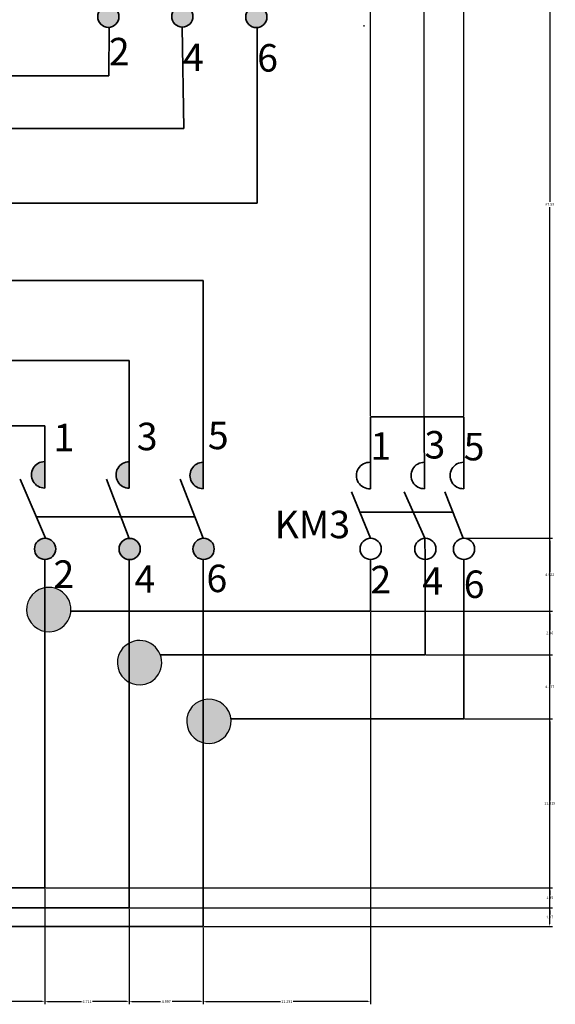
# Model space of a CAD drawing. Units: inches. Extents: x 237 to 313, y 343 to 451.
# Tile 2 of 6: x 277 to 313, y 343 to 410. Entities that reach past the tile are written whole.
import ezdxf

# ---------------------------------------------------------------- set-up
doc = ezdxf.new("R2010")
doc.units = ezdxf.units.IN
doc.header["$MEASUREMENT"] = 0
doc.layers.get('0').update_dxf_attribs({"color": 240})
for name, color, linetype, lineweight in [('A-ANNO-DIMS', 2, 'Continuous', 18), ('E-ANNO-TEXT', 7, 'Continuous', 25), ('E-DEVC', 4, 'Continuous', 35), ('E-PATT', 8, 'Continuous', 13), ('E-WIRE', 7, 'Continuous', 35), ('E-WIRE-JUNC', 7, 'Continuous', 25)]:
    doc.layers.add(name, color=color, linetype=linetype, lineweight=lineweight)
doc.styles.get("Standard").update_dxf_attribs({"font": 'arial.ttf'})
doc.dimstyles.get("Standard").update_dxf_attribs({"dimtxt": 0.18, "dimasz": 0.18, "dimexe": 0.18, "dimexo": 0.0625, "dimgap": 0.09, "dimtad": 0, "dimtih": 1, "dimtoh": 1, "dimdec": 4, "dimzin": 0, "dimdsep": 46, "dimtxsty": 'Standard', "dimcen": 0.09, "dimadec": 0, "dimazin": 0, "dimtfac": 1, "dimtdec": 4, "dimtofl": 0, "dimtmove": 0, "dimatfit": 3, "dimfxl": 1, "dimtolj": 1, "dimtzin": 0, "dimarcsym": 0})

# ---------------------------------------------------------------- blocks, each defined once
blk = doc.blocks.new('CONTACTOR-3P-NO')
h = blk.add_hatch(color=256)
h.dxf.hatch_style = 1
h.paths.add_polyline_path([(1.637, 4.965, 1), (1.637, 3.177)])
h.paths.add_polyline_path([(6.637, 4.953, 1), (6.637, 3.166)])
h.paths.add_polyline_path([(11.637, 4.931, 1), (11.637, 3.144)])
h = blk.add_hatch(color=256)
h.dxf.hatch_style = 1
h.paths.add_polyline_path([(2.354, 0.734, 1), (0.92, 0.734, 1)])
h.paths.add_polyline_path([(5.92, 0.749, 1), (7.354, 0.749, 1)])
h.paths.add_polyline_path([(10.92, 0.717, 1), (12.354, 0.717, 1)])
for p, q in [((1.414, 1.415), (0, 3.965)), ((6.423, 1.433), (4.991, 3.965)), ((11.461, 1.412), (9.739, 3.965))]:
    blk.add_line(p, q)
for centre in [(1.637, 0.734), (6.637, 0.749), (11.637, 0.717)]:
    blk.add_circle(centre, 0.717)
for centre in [(1.637, 4.071), (6.637, 4.06), (11.637, 4.037)]:
    blk.add_arc(centre, 0.894, 90, 270)
blk = doc.blocks.new('*D3')
at = {"layer": 'A-ANNO-DIMS', "color": 0, "lineweight": -2, "transparency": 16777216}
for p, q in [((242.3, 363.785), (242.3, 451.078)), ((242.48, 450.898), (274.084, 450.898)), ((306.476, 450.898), (274.872, 450.898)), ((306.656, 382.738), (306.656, 451.078))]:
    blk.add_line(p, q, dxfattribs=at)
at = {"layer": 'A-ANNO-DIMS', "color": 0, "lineweight": 35, "transparency": 16777216}
for points in [[(242.48, 450.928), (242.48, 450.868), (242.3, 450.898)], [(306.476, 450.928), (306.476, 450.868), (306.656, 450.898)]]:
    blk.add_solid(points, dxfattribs=at)
at = {"layer": 'Defpoints', "color": 0, "lineweight": 35, "transparency": 16777216}
for p in [(306.656, 450.898), (306.656, 382.675), (242.3, 363.723)]:
    blk.add_point(p, dxfattribs=at)
at = {"layer": 'A-ANNO-DIMS', "color": 0, "transparency": 16777216, "insert": (274.478, 450.898), "char_height": 0.18, "attachment_point": 5}
blk.add_mtext('\\A1;64.36', dxfattribs=at)
blk = doc.blocks.new('*D4')
at = {"layer": 'A-ANNO-DIMS', "color": 0, "lineweight": -2, "transparency": 16777216}
for p, q in [((258.115, 445.823), (312.65, 445.823)), ((312.47, 445.643), (312.47, 397.21)), ((312.47, 348.414), (312.47, 396.846)), ((289.124, 348.234), (312.65, 348.234))]:
    blk.add_line(p, q, dxfattribs=at)
at = {"layer": 'A-ANNO-DIMS', "color": 0, "lineweight": 35, "transparency": 16777216}
for points in [[(312.44, 445.643), (312.5, 445.643), (312.47, 445.823)], [(312.44, 348.414), (312.5, 348.414), (312.47, 348.234)]]:
    blk.add_solid(points, dxfattribs=at)
at = {"layer": 'Defpoints', "color": 0, "lineweight": 35, "transparency": 16777216}
for p in [(258.052, 445.823), (289.062, 348.234), (312.47, 348.234)]:
    blk.add_point(p, dxfattribs=at)
at = {"layer": 'A-ANNO-DIMS', "color": 0, "transparency": 16777216, "insert": (312.47, 397.028), "char_height": 0.18, "attachment_point": 5}
blk.add_mtext('\\A1;97.59', dxfattribs=at)
blk = doc.blocks.new('*D10')
at = {"layer": 'A-ANNO-DIMS', "color": 0, "lineweight": -2, "transparency": 16777216}
for p, q in [((300.353, 382.738), (300.353, 451.078)), ((300.533, 450.898), (301.848, 450.898)), ((303.809, 450.898), (302.495, 450.898)), ((303.989, 382.738), (303.989, 451.078))]:
    blk.add_line(p, q, dxfattribs=at)
at = {"layer": 'A-ANNO-DIMS', "color": 0, "lineweight": 35, "transparency": 16777216}
for points in [[(300.533, 450.928), (300.533, 450.868), (300.353, 450.898)], [(303.809, 450.928), (303.809, 450.868), (303.989, 450.898)]]:
    blk.add_solid(points, dxfattribs=at)
at = {"layer": 'Defpoints', "color": 0, "lineweight": 35, "transparency": 16777216}
for p in [(303.989, 450.898), (300.353, 382.675), (303.989, 382.675)]:
    blk.add_point(p, dxfattribs=at)
at = {"layer": 'A-ANNO-DIMS', "color": 0, "transparency": 16777216, "insert": (302.171, 450.898), "char_height": 0.18, "attachment_point": 5}
blk.add_mtext('\\A1;3.64', dxfattribs=at)
blk = doc.blocks.new('*D11')
at = {"layer": 'A-ANNO-DIMS', "color": 0, "lineweight": -2, "transparency": 16777216}
for p, q in [((303.989, 382.738), (303.989, 451.078)), ((304.169, 450.898), (304.928, 450.898)), ((306.476, 450.898), (305.718, 450.898)), ((306.656, 382.738), (306.656, 451.078))]:
    blk.add_line(p, q, dxfattribs=at)
at = {"layer": 'A-ANNO-DIMS', "color": 0, "lineweight": 35, "transparency": 16777216}
for points in [[(304.169, 450.928), (304.169, 450.868), (303.989, 450.898)], [(306.476, 450.928), (306.476, 450.868), (306.656, 450.898)]]:
    blk.add_solid(points, dxfattribs=at)
at = {"layer": 'Defpoints', "color": 0, "lineweight": 35, "transparency": 16777216}
for p in [(306.656, 450.898), (303.989, 382.675), (306.656, 382.675)]:
    blk.add_point(p, dxfattribs=at)
at = {"layer": 'A-ANNO-DIMS', "color": 0, "transparency": 16777216, "insert": (305.323, 450.898), "char_height": 0.18, "attachment_point": 5}
blk.add_mtext('\\A1;2.667', dxfattribs=at)
blk = doc.blocks.new('*D14')
at = {"layer": 'A-ANNO-DIMS', "color": 0, "lineweight": -2, "transparency": 16777216}
for p, q in [((278.353, 350.796), (278.353, 342.979)), ((259.191, 348.171), (259.191, 342.979)), ((259.371, 343.159), (268.317, 343.159)), ((278.173, 343.159), (269.227, 343.159))]:
    blk.add_line(p, q, dxfattribs=at)
at = {"layer": 'A-ANNO-DIMS', "color": 0, "lineweight": 35, "transparency": 16777216}
for points in [[(259.371, 343.189), (259.371, 343.129), (259.191, 343.159)], [(278.173, 343.189), (278.173, 343.129), (278.353, 343.159)]]:
    blk.add_solid(points, dxfattribs=at)
at = {"layer": 'Defpoints', "color": 0, "lineweight": 35, "transparency": 16777216}
for p in [(278.353, 350.859), (259.191, 348.234), (278.353, 343.159)]:
    blk.add_point(p, dxfattribs=at)
at = {"layer": 'A-ANNO-DIMS', "color": 0, "transparency": 16777216, "insert": (268.772, 343.159), "char_height": 0.18, "attachment_point": 5}
blk.add_mtext('\\A1;19.163', dxfattribs=at)
blk = doc.blocks.new('*D15')
at = {"layer": 'A-ANNO-DIMS', "color": 0, "lineweight": -2, "transparency": 16777216}
for p, q in [((278.353, 350.796), (278.353, 342.979)), ((284.064, 349.444), (284.064, 342.979)), ((278.533, 343.159), (280.833, 343.159)), ((283.884, 343.159), (281.585, 343.159))]:
    blk.add_line(p, q, dxfattribs=at)
at = {"layer": 'A-ANNO-DIMS', "color": 0, "lineweight": 35, "transparency": 16777216}
for points in [[(278.533, 343.189), (278.533, 343.129), (278.353, 343.159)], [(283.884, 343.189), (283.884, 343.129), (284.064, 343.159)]]:
    blk.add_solid(points, dxfattribs=at)
at = {"layer": 'Defpoints', "color": 0, "lineweight": 35, "transparency": 16777216}
for p in [(278.353, 350.859), (284.064, 349.506), (284.064, 343.159)]:
    blk.add_point(p, dxfattribs=at)
at = {"layer": 'A-ANNO-DIMS', "color": 0, "transparency": 16777216, "insert": (281.209, 343.159), "char_height": 0.18, "attachment_point": 5}
blk.add_mtext('\\A1;5.711', dxfattribs=at)
blk = doc.blocks.new('*D16')
at = {"layer": 'A-ANNO-DIMS', "color": 0, "lineweight": -2, "transparency": 16777216}
for p, q in [((284.064, 349.444), (284.064, 342.979)), ((289.062, 348.171), (289.062, 342.979)), ((284.244, 343.159), (286.166, 343.159)), ((288.882, 343.159), (286.96, 343.159))]:
    blk.add_line(p, q, dxfattribs=at)
at = {"layer": 'A-ANNO-DIMS', "color": 0, "lineweight": 35, "transparency": 16777216}
for points in [[(284.244, 343.189), (284.244, 343.129), (284.064, 343.159)], [(288.882, 343.189), (288.882, 343.129), (289.062, 343.159)]]:
    blk.add_solid(points, dxfattribs=at)
at = {"layer": 'Defpoints', "color": 0, "lineweight": 35, "transparency": 16777216}
for p in [(284.064, 349.506), (289.062, 348.234), (289.062, 343.159)]:
    blk.add_point(p, dxfattribs=at)
at = {"layer": 'A-ANNO-DIMS', "color": 0, "transparency": 16777216, "insert": (286.563, 343.159), "char_height": 0.18, "attachment_point": 5}
blk.add_mtext('\\A1;4.997', dxfattribs=at)
blk = doc.blocks.new('*D17')
at = {"layer": 'A-ANNO-DIMS', "color": 0, "lineweight": -2, "transparency": 16777216}
for p, q in [((300.353, 369.487), (300.353, 342.979)), ((289.062, 348.171), (289.062, 342.979)), ((289.242, 343.159), (294.269, 343.159)), ((300.173, 343.159), (295.145, 343.159))]:
    blk.add_line(p, q, dxfattribs=at)
at = {"layer": 'A-ANNO-DIMS', "color": 0, "lineweight": 35, "transparency": 16777216}
for points in [[(289.242, 343.189), (289.242, 343.129), (289.062, 343.159)], [(300.173, 343.189), (300.173, 343.129), (300.353, 343.159)]]:
    blk.add_solid(points, dxfattribs=at)
at = {"layer": 'Defpoints', "color": 0, "lineweight": 35, "transparency": 16777216}
for p in [(300.353, 369.549), (289.062, 348.234), (300.353, 343.159)]:
    blk.add_point(p, dxfattribs=at)
at = {"layer": 'A-ANNO-DIMS', "color": 0, "transparency": 16777216, "insert": (294.707, 343.159), "char_height": 0.18, "attachment_point": 5}
blk.add_mtext('\\A1;11.291', dxfattribs=at)
blk = doc.blocks.new('*D18')
at = {"layer": 'A-ANNO-DIMS', "color": 0, "lineweight": -2, "transparency": 16777216}
for p, q in [((306.741, 374.471), (312.65, 374.471)), ((312.47, 374.291), (312.47, 372.192)), ((312.47, 369.729), (312.47, 371.828)), ((300.415, 369.549), (312.65, 369.549))]:
    blk.add_line(p, q, dxfattribs=at)
at = {"layer": 'A-ANNO-DIMS', "color": 0, "lineweight": 35, "transparency": 16777216}
for points in [[(312.44, 374.291), (312.5, 374.291), (312.47, 374.471)], [(312.44, 369.729), (312.5, 369.729), (312.47, 369.549)]]:
    blk.add_solid(points, dxfattribs=at)
at = {"layer": 'Defpoints', "color": 0, "lineweight": 35, "transparency": 16777216}
for p in [(306.678, 374.471), (300.353, 369.549), (312.47, 369.549)]:
    blk.add_point(p, dxfattribs=at)
at = {"layer": 'A-ANNO-DIMS', "color": 0, "transparency": 16777216, "insert": (312.47, 372.01), "char_height": 0.18, "attachment_point": 5}
blk.add_mtext('\\A1;4.922', dxfattribs=at)
blk = doc.blocks.new('*D19')
at = {"layer": 'A-ANNO-DIMS', "color": 0, "lineweight": -2, "transparency": 16777216}
for p, q in [((300.415, 369.549), (312.65, 369.549)), ((312.47, 369.369), (312.47, 368.252)), ((312.47, 366.772), (312.47, 367.888)), ((304.107, 366.592), (312.65, 366.592))]:
    blk.add_line(p, q, dxfattribs=at)
at = {"layer": 'A-ANNO-DIMS', "color": 0, "lineweight": 35, "transparency": 16777216}
for points in [[(312.44, 369.369), (312.5, 369.369), (312.47, 369.549)], [(312.44, 366.772), (312.5, 366.772), (312.47, 366.592)]]:
    blk.add_solid(points, dxfattribs=at)
at = {"layer": 'Defpoints', "color": 0, "lineweight": 35, "transparency": 16777216}
for p in [(300.353, 369.549), (304.045, 366.592), (312.47, 366.592)]:
    blk.add_point(p, dxfattribs=at)
at = {"layer": 'A-ANNO-DIMS', "color": 0, "transparency": 16777216, "insert": (312.47, 368.07), "char_height": 0.18, "attachment_point": 5}
blk.add_mtext('\\A1;2.96', dxfattribs=at)
blk = doc.blocks.new('*D20')
at = {"layer": 'A-ANNO-DIMS', "color": 0, "lineweight": -2, "transparency": 16777216}
for p, q in [((304.107, 366.592), (312.65, 366.592)), ((312.47, 366.412), (312.47, 364.615)), ((312.47, 362.454), (312.47, 364.251)), ((306.719, 362.274), (312.65, 362.274))]:
    blk.add_line(p, q, dxfattribs=at)
at = {"layer": 'A-ANNO-DIMS', "color": 0, "lineweight": 35, "transparency": 16777216}
for points in [[(312.44, 366.412), (312.5, 366.412), (312.47, 366.592)], [(312.44, 362.454), (312.5, 362.454), (312.47, 362.274)]]:
    blk.add_solid(points, dxfattribs=at)
at = {"layer": 'Defpoints', "color": 0, "lineweight": 35, "transparency": 16777216}
for p in [(304.045, 366.592), (306.656, 362.274), (312.47, 362.274)]:
    blk.add_point(p, dxfattribs=at)
at = {"layer": 'A-ANNO-DIMS', "color": 0, "transparency": 16777216, "insert": (312.47, 364.433), "char_height": 0.18, "attachment_point": 5}
blk.add_mtext('\\A1;4.317', dxfattribs=at)
blk = doc.blocks.new('*D21')
at = {"layer": 'A-ANNO-DIMS', "color": 0, "lineweight": -2, "transparency": 16777216}
for p, q in [((306.719, 362.274), (312.65, 362.274)), ((312.47, 362.094), (312.47, 356.748)), ((312.47, 351.039), (312.47, 356.385)), ((278.416, 350.859), (312.65, 350.859))]:
    blk.add_line(p, q, dxfattribs=at)
at = {"layer": 'A-ANNO-DIMS', "color": 0, "lineweight": 35, "transparency": 16777216}
for points in [[(312.44, 362.094), (312.5, 362.094), (312.47, 362.274)], [(312.44, 351.039), (312.5, 351.039), (312.47, 350.859)]]:
    blk.add_solid(points, dxfattribs=at)
at = {"layer": 'Defpoints', "color": 0, "lineweight": 35, "transparency": 16777216}
for p in [(306.656, 362.274), (278.353, 350.859), (312.47, 350.859)]:
    blk.add_point(p, dxfattribs=at)
at = {"layer": 'A-ANNO-DIMS', "color": 0, "transparency": 16777216, "insert": (312.47, 356.567), "char_height": 0.18, "attachment_point": 5}
blk.add_mtext('\\A1;11.415', dxfattribs=at)
blk = doc.blocks.new('*D22')
at = {"layer": 'A-ANNO-DIMS', "color": 0, "lineweight": -2, "transparency": 16777216}
for p, q in [((278.416, 350.859), (312.65, 350.859)), ((312.47, 350.679), (312.47, 350.364)), ((312.47, 349.686), (312.47, 350.001)), ((284.127, 349.506), (312.65, 349.506))]:
    blk.add_line(p, q, dxfattribs=at)
at = {"layer": 'A-ANNO-DIMS', "color": 0, "lineweight": 35, "transparency": 16777216}
for points in [[(312.44, 350.679), (312.5, 350.679), (312.47, 350.859)], [(312.44, 349.686), (312.5, 349.686), (312.47, 349.506)]]:
    blk.add_solid(points, dxfattribs=at)
at = {"layer": 'Defpoints', "color": 0, "lineweight": 35, "transparency": 16777216}
for p in [(278.353, 350.859), (284.064, 349.506), (312.47, 349.506)]:
    blk.add_point(p, dxfattribs=at)
at = {"layer": 'A-ANNO-DIMS', "color": 0, "transparency": 16777216, "insert": (312.47, 350.183), "char_height": 0.18, "attachment_point": 5}
blk.add_mtext('\\A1;1.35', dxfattribs=at)
blk = doc.blocks.new('*D23')
at = {"layer": 'A-ANNO-DIMS', "color": 0, "lineweight": -2, "transparency": 16777216}
for p, q in [((284.127, 349.506), (312.65, 349.506)), ((312.47, 349.326), (312.47, 349.05)), ((312.47, 348.414), (312.47, 348.69)), ((289.124, 348.234), (312.65, 348.234))]:
    blk.add_line(p, q, dxfattribs=at)
at = {"layer": 'A-ANNO-DIMS', "color": 0, "lineweight": 35, "transparency": 16777216}
for points in [[(312.44, 349.326), (312.5, 349.326), (312.47, 349.506)], [(312.44, 348.414), (312.5, 348.414), (312.47, 348.234)]]:
    blk.add_solid(points, dxfattribs=at)
at = {"layer": 'Defpoints', "color": 0, "lineweight": 35, "transparency": 16777216}
for p in [(284.064, 349.506), (289.062, 348.234), (312.47, 348.234)]:
    blk.add_point(p, dxfattribs=at)
at = {"layer": 'A-ANNO-DIMS', "color": 0, "transparency": 16777216, "insert": (312.47, 348.87), "char_height": 0.18, "attachment_point": 5}
blk.add_mtext('\\A1;1.27', dxfattribs=at)

msp = doc.modelspace()

# ---------------------------------------------------------------- hatches: boundary and pattern name
at = {"layer": 'E-PATT'}
h = msp.add_hatch(color=256, dxfattribs=at)
h.dxf.hatch_style = 1
h.paths.add_polyline_path([(278.3534, 379.6524, 1.0110136), (278.3534, 377.8655)])
h.paths.add_polyline_path([(284.0644, 379.6407, 1.0041673), (284.0644, 377.8536)])
h.paths.add_polyline_path([(289.0615, 379.6052, 1.0065142), (289.0615, 377.8181)])
h = msp.add_hatch(color=256, dxfattribs=at)
h.dxf.hatch_style = 1
h.paths.add_polyline_path([(277.6585, 373.7542, 1), (279.0922, 373.7542, 1)])
h.paths.add_polyline_path([(283.3695, 373.7487, 1), (284.8032, 373.7487, 1)])
h.paths.add_polyline_path([(289.8002, 373.7542, 1), (288.3666, 373.7542, 1)])
h = msp.add_hatch(color=256, dxfattribs=at)
h.dxf.hatch_style = 1
h.paths.add_polyline_path([(280.0786, 370.0264), (277.1724, 369.2822, 0.4142136), (278.9976, 368.2012, 0.4142136)])
h.paths.add_polyline_path([(280.0786, 370.0264, 0.4142136), (278.2534, 371.1074, 0.4142136), (277.1724, 369.2822)])
h.paths.add_polyline_path([(285.1284, 364.6098, 0.4142136), (286.2094, 366.435), (283.3032, 365.6908, 0.4142136)])
h.paths.add_polyline_path([(286.2094, 366.435, 0.4142136), (284.3842, 367.516, 0.4142136), (283.3032, 365.6908)])
h.paths.add_polyline_path([(290.8939, 362.4733, 0.4142136), (289.0687, 363.5543, 0.4142136), (287.9877, 361.7291)])
h.paths.add_polyline_path([(289.8129, 360.6481, 0.4142136), (290.8939, 362.4733), (287.9877, 361.7291, 0.4142136)])

# ---------------------------------------------------------------- linework, layer by layer
at = {"layer": 'E-DEVC'}
for p, q in [((299.9631, 409.1047), (299.8791, 409.1047)), ((278.3965, 374.4708), (276.6917, 378.4537)), ((284.063, 374.4651), (282.5289, 378.4537)), ((289.0532, 374.4704), (287.4926, 378.4537)), ((300.3616, 374.471), (299.0722, 377.6008)), ((304.0363, 374.4704), (302.6377, 377.6008)), ((306.629, 374.4694), (305.3927, 377.6008)), ((305.9288, 376.2428), (299.6317, 376.2428)), ((288.4889, 375.9107), (277.7775, 375.917))]:
    msp.add_line(p, q, dxfattribs=at)
for centre in [(278.3753, 373.7542), (284.0863, 373.7487), (289.0834, 373.7542), (300.3748, 373.7542), (304.0664, 373.7542), (306.6783, 373.7542)]:
    msp.add_circle(centre, 0.7168, dxfattribs=at)
for centre, start, end in [((278.3436, 378.7589), 90, 270.627572), ((284.0607, 378.7471), 90, 270.23827), ((289.0557, 378.7116), 89.627979, 270.372021), ((300.3001, 378.7116), 86.613991, 273.386009), ((303.9916, 378.7116), 89.012547, 271.641897), ((306.6337, 378.7116), 88.544288, 271.455712)]:
    msp.add_arc(centre, 0.8935, start, end, dxfattribs=at)
at = {"layer": 'E-WIRE'}
for p, q in [((282.7144, 409), (282.6795, 405.7183)), ((287.6421, 409.0119), (287.7431, 402.163)), ((292.7019, 408.9818), (292.7062, 397.1148)), ((259.4968, 405.7183), (282.6795, 405.7183)), ((254.4968, 402.163), (287.7431, 402.163)), ((249.4968, 397.1148), (292.7062, 397.1148)), ((259.4968, 391.8904), (289.0615, 391.8904)), ((289.0615, 391.8904), (289.0615, 377.8181)), ((254.4968, 386.4864), (284.0644, 386.4864)), ((284.0644, 386.4864), (284.0644, 377.8536)), ((300.3529, 377.8197), (300.3529, 382.675)), ((300.3529, 382.675), (306.6564, 382.675)), ((304.0172, 377.8185), (303.9895, 382.675)), ((306.6564, 382.675), (306.6564, 377.8184)), ((249.4968, 382.0712), (278.3534, 382.0712)), ((278.3534, 382.0712), (278.3534, 377.8655)), ((304.0445, 373.0378), (304.0363, 374.4704)), ((278.3534, 373.0378), (278.3534, 350.8589)), ((284.0644, 373.0322), (284.0644, 349.5062)), ((289.0615, 373.0378), (289.0615, 348.2337)), ((300.3529, 369.549), (300.3529, 373.0378)), ((304.0445, 366.5916), (304.0445, 373.0378)), ((306.6564, 362.2743), (306.6564, 373.0378)), ((284.0644, 370.8013), (284.0644, 366.0525)), ((280.1218, 369.549), (300.3529, 369.549)), ((286.1601, 366.5916), (304.0445, 366.5916)), ((290.9308, 362.2743), (306.6564, 362.2743)), ((248.0836, 350.8589), (278.3534, 350.8589)), ((252.9002, 349.5062), (284.0644, 349.5062)), ((259.1907, 348.2337), (289.0615, 348.2337))]:
    msp.add_line(p, q, dxfattribs=at)
at = {"layer": 'E-WIRE-JUNC'}
for points in [[(278.2534, 371.1074, 1), (278.9976, 368.2012, 1)], [(284.3842, 367.516, 1), (285.1284, 364.6098, 1)], [(289.0687, 363.5543, 1), (289.8129, 360.6481, 1)]]:
    msp.add_lwpolyline(points, format="xyb", close=True, dxfattribs=at)

# ---------------------------------------------------------------- block references
at = {"layer": 'E-DEVC'}
msp.add_blockref('CONTACTOR-3P-NO', (281.0109, 408.98), dxfattribs=at)

# ---------------------------------------------------------------- texts
at = {"layer": 'E-ANNO-TEXT'}
for s, height, p in [('2', 1.8564, (282.687, 406.4281)), ('4', 1.8564, (287.686, 406.0373)), ('6', 1.8564, (292.703, 406.0062)), ('1', 1.8564, (278.9453, 380.3524)), ('3', 1.8564, (284.5717, 380.4212)), ('5', 1.8564, (289.3713, 380.4901)), ('1', 1.8564, (300.3529, 379.7747)), ('3', 1.8564, (304.0056, 379.8606)), ('5', 1.8564, (306.6564, 379.7356)), ('KM3', 1.85645, (293.8817, 374.4742)), ('2', 1.8564, (278.9422, 371.1205)), ('4', 1.8564, (284.4171, 370.7896)), ('6', 1.8564, (289.2752, 370.8323)), ('2', 1.8564, (300.3529, 370.749)), ('4', 1.8564, (303.8574, 370.6523)), ('6', 1.8564, (306.6564, 370.4363))]:
    msp.add_text(s, height=height, dxfattribs=at).set_placement(p)

# ---------------------------------------------------------------- dimensions: what is measured, and where the dimension line sits
at = {"layer": 'A-ANNO-DIMS'}
for base, p1, p2, override, picture, middle in [((306.6564, 450.8976), (242.3002, 363.7227), (306.6564, 382.675), {"dimdec": 2, "dimlfac": 1, "dimrnd": 0, "dimzin": 0, "dimdsep": 46, "dimlunit": 2}, '*D3', (274.4783, 450.8976)), ((303.9895, 450.8976), (300.3529, 382.675), (303.9895, 382.675), {"dimdec": 2, "dimlfac": 1, "dimrnd": 0, "dimzin": 0, "dimdsep": 46, "dimlunit": 2}, '*D10', (302.1712, 450.8976)), ((306.6564, 450.8976), (303.9895, 382.675), (306.6564, 382.675), {"dimdec": 3, "dimlfac": 1, "dimrnd": 0, "dimzin": 0, "dimdsep": 46, "dimlunit": 2}, '*D11', (305.3229, 450.8976)), ((300.3529, 343.1587), (289.0615, 348.2337), (300.3529, 369.549), {"dimdec": 3, "dimlfac": 1, "dimrnd": 0, "dimzin": 0, "dimdsep": 46, "dimlunit": 2}, '*D17', (294.7072, 343.1587)), ((278.3534, 343.1587), (259.1907, 348.2337), (278.3534, 350.8589), {"dimdec": 3, "dimlfac": 1, "dimrnd": 0, "dimzin": 0, "dimdsep": 46, "dimlunit": 2}, '*D14', (268.7721, 343.1587)), ((284.0644, 343.1587), (278.3534, 350.8589), (284.0644, 349.5062), {"dimdec": 3, "dimlfac": 1, "dimrnd": 0, "dimzin": 0, "dimdsep": 46, "dimlunit": 2}, '*D15', (281.2089, 343.1587)), ((289.0615, 343.1587), (284.0644, 349.5062), (289.0615, 348.2337), {"dimdec": 3, "dimlfac": 1, "dimrnd": 0, "dimzin": 0, "dimdsep": 46, "dimlunit": 2}, '*D16', (286.563, 343.1587))]:
    dim = msp.add_linear_dim(base=base, p1=p1, p2=p2, dimstyle='Standard', override=override, dxfattribs=at)
    dim.commit()
    dim.dimension.update_dxf_attribs({"geometry": picture, "text_midpoint": middle})
for base, p1, p2, override, picture, middle in [((312.4701, 348.2337), (258.0525, 445.8226), (289.0615, 348.2337), {"dimdec": 2, "dimlfac": 1, "dimrnd": 0, "dimzin": 0, "dimdsep": 46, "dimlunit": 2}, '*D4', (312.4701, 397.0282)), ((312.4701, 369.549), (306.6783, 374.4711), (300.3529, 369.549), {"dimdec": 3, "dimlfac": 1, "dimrnd": 0, "dimzin": 0, "dimdsep": 46, "dimlunit": 2}, '*D18', (312.4701, 372.01)), ((312.4701, 366.5916), (300.3529, 369.549), (304.0445, 366.5916), {"dimdec": 2, "dimlfac": 1, "dimrnd": 0, "dimzin": 0, "dimdsep": 46, "dimlunit": 2}, '*D19', (312.4701, 368.0703)), ((312.4701, 362.2743), (304.0445, 366.5916), (306.6564, 362.2743), {"dimdec": 3, "dimlfac": 1, "dimrnd": 0, "dimzin": 0, "dimdsep": 46, "dimlunit": 2}, '*D20', (312.4701, 364.4329)), ((312.4701, 350.8589), (306.6564, 362.2743), (278.3534, 350.8589), {"dimdec": 3, "dimlfac": 1, "dimrnd": 0, "dimzin": 0, "dimdsep": 46, "dimlunit": 2}, '*D21', (312.4701, 356.5666)), ((312.4701, 349.5062), (278.3534, 350.8589), (284.0644, 349.5062), {"dimdec": 2, "dimlfac": 1, "dimrnd": 0, "dimzin": 0, "dimdsep": 46, "dimlunit": 2}, '*D22', (312.4701, 350.1825)), ((312.4701, 348.2337), (284.0644, 349.5062), (289.0615, 348.2337), {"dimdec": 2, "dimlfac": 1, "dimrnd": 0, "dimzin": 0, "dimdsep": 46, "dimlunit": 2}, '*D23', (312.4701, 348.8699))]:
    dim = msp.add_linear_dim(base=base, p1=p1, p2=p2, angle=90, dimstyle='Standard', override=override, dxfattribs=at)
    dim.commit()
    dim.dimension.update_dxf_attribs({"geometry": picture, "text_midpoint": middle})

doc.saveas('drawing.dxf')
